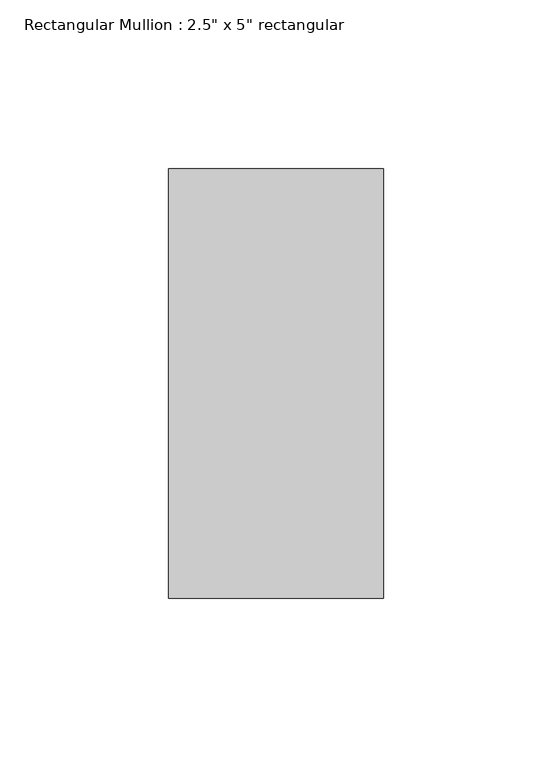
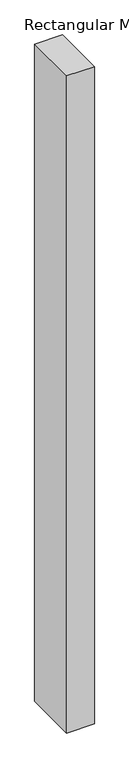
"""IFC4 building model written with IfcOpenShell, lengths in millimetres: member geometry."""

from ifc_helpers import new_model, si_unit, frame, origin, place, context, project, spatial, polyline, outline, extrude, source, transform, mapped, element, save


def member_e65a551c(model_context):
    return source(origin(), model_context, "Body", "SweptSolid", [
        extrude(outline(polyline([(0.0, 63.5), (0.0, -63.5), (-63.5, -63.5), (-63.5, 63.5), (0.0, 63.5)])), frame((0.0, 0.0, -1593.2699234), z_axis=(0.0, 0.0, 1.0), x_axis=(1.0, 0.0, 0.0)), (0.0, 0.0, 1.0), 1593.2699234),
    ])


if __name__ == "__main__":
    model = new_model("IFC4")
    model_context = context("Model", 3, world=origin())
    ifc_project = project(units=[si_unit("LENGTHUNIT", "METRE", prefix="MILLI")], contexts=[model_context])
    site = spatial("IfcSite", under=ifc_project)
    building = spatial("IfcBuilding", under=site)
    placement = place(None, origin())
    member_shape = member_e65a551c(model_context)
    element("IfcMember", 1, ObjectType="Rectangular Mullion : 2.5\" x 5\" rectangular", at=placement, inside=building, context=model_context, shape_type="MappedRepresentation", body=[
        mapped(member_shape, transform((0.0, 0.0, 0.0), x_axis=(1.0, 0.0, 0.0), y_axis=(0.0, 1.0, 0.0), z_axis=(0.0, 0.0, 1.0))),
    ])
    save(model, "model.ifc")

# Revit data of these elements
# Type "Rectangular Mullion : 2.5\" x 5\" rectangular"
#   built-in parameter 1007304 = 0.416667 (stored number, unit not read)
#   built-in parameter 1007301 = 0.104167 (stored number, unit not read)
#   built-in parameter 1007300 = 0.104167 (stored number, unit not read)
# Element 1 (IfcMember, "Rectangular Mullion : 2.5\" x 5\" rectangular")
#   Materials on its faces: "Aluminum"
# Materials
#   "Aluminum": class "Metal", colour RGB 247 247 247, transparency 0, Description = "Aluminum 6061", Cost = 0
